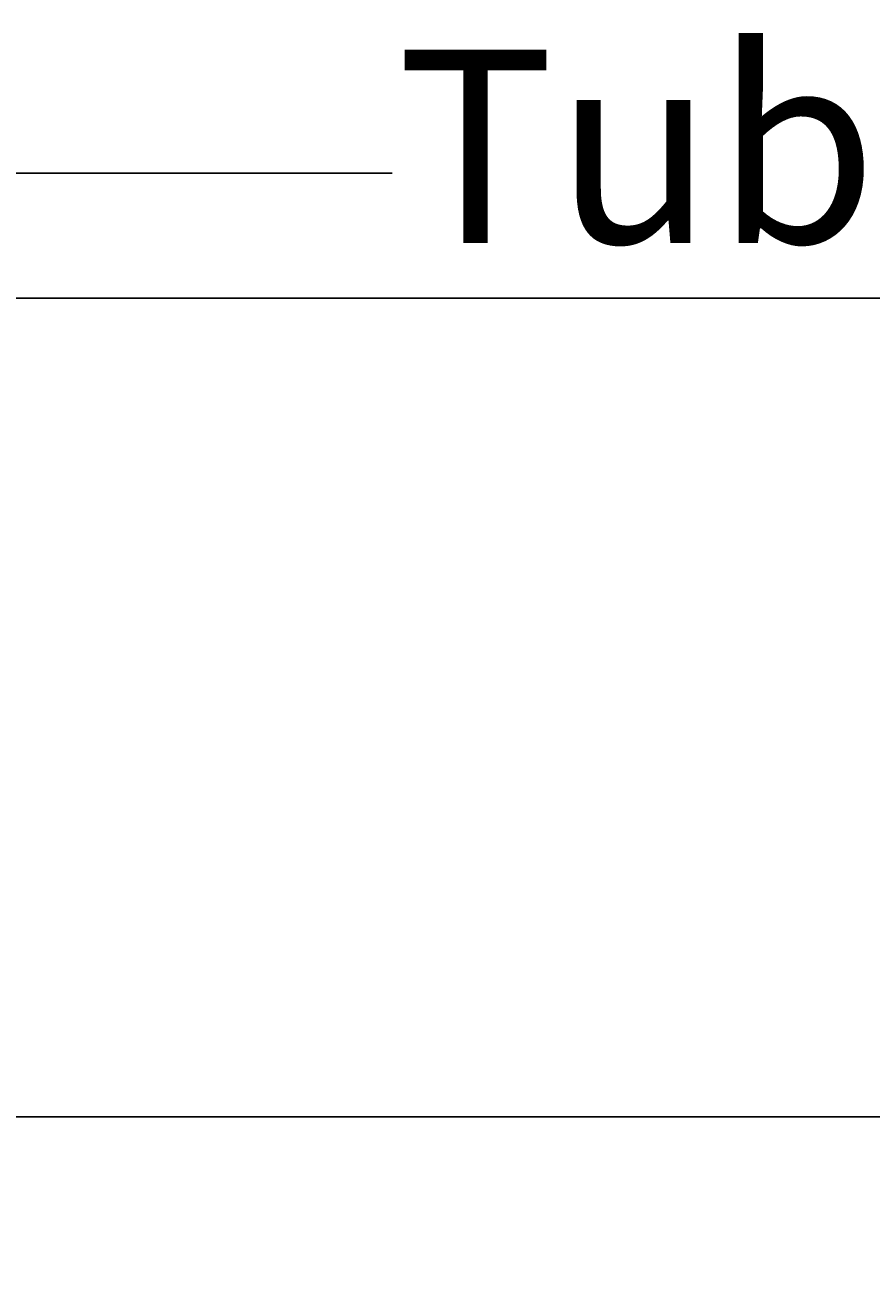
# Model space of a CAD drawing. Units: inches. Extents: x -12 to 334, y -10 to 186.
# Tile 26 of 77: x 88 to 106, y 135 to 160. Entities that reach past the tile are written whole.
import ezdxf
from ezdxf import colors
from ezdxf.entities.mleader import LeaderData, LeaderLine
from ezdxf.math import Vec2, Vec3

# ---------------------------------------------------------------- set-up
doc = ezdxf.new("R2010")
doc.units = ezdxf.units.IN
doc.header["$MEASUREMENT"] = 0
doc.layers.add('M-ANNO-TEXT', color=3, linetype='Continuous', lineweight=25)
doc.layers.add('M-DIMS', color=2, linetype='Continuous', lineweight=18)
doc.styles.get("Standard").update_dxf_attribs({"font": 'arial.ttf'})
doc.dimstyles.get("Standard").update_dxf_attribs({"dimtxt": 0.18, "dimasz": 0.18, "dimexe": 0.18, "dimexo": 0.0625, "dimgap": 0.09, "dimtad": 0, "dimtih": 1, "dimtoh": 1, "dimdec": 4, "dimzin": 0, "dimdsep": 46, "dimtxsty": 'Standard', "dimcen": 0.09, "dimadec": 0, "dimazin": 0, "dimtfac": 1, "dimtdec": 4, "dimtofl": 0, "dimtmove": 0, "dimatfit": 3, "dimfxl": 1, "dimtolj": 1, "dimtzin": 0, "dimarcsym": 0})

# ---------------------------------------------------------------- blocks, each defined once
blk = doc.blocks.new('*D15')
at = {"layer": 'Defpoints', "color": 0, "transparency": 16777216}
for p in [(106.177, 169.385), (86.888, 109.058), (106.177, 102.896)]:
    blk.add_point(p, dxfattribs=at)
at = {"layer": 'M-DIMS', "color": 0, "lineweight": -2, "transparency": 16777216}
for p, q in [((86.888, 109.121), (86.888, 169.565)), ((106.177, 102.958), (106.177, 169.565)), ((87.068, 169.385), (96.147, 169.385)), ((105.997, 169.385), (96.918, 169.385))]:
    blk.add_line(p, q, dxfattribs=at)
at = {"layer": 'M-DIMS', "color": 0, "transparency": 16777216}
for points in [[(87.068, 169.415), (87.068, 169.355), (86.888, 169.385)], [(105.997, 169.415), (105.997, 169.355), (106.177, 169.385)]]:
    blk.add_solid(points, dxfattribs=at)
at = {"layer": 'M-DIMS', "color": 0, "transparency": 16777216, "insert": (96.532, 169.385), "char_height": 0.18, "attachment_point": 5}
blk.add_mtext('\\A1;19.29', dxfattribs=at)
blk = doc.blocks.new('*D22')
at = {"layer": 'Defpoints', "color": 0, "transparency": 16777216}
for p in [(190.342, 154.835), (-11.174, 137.887), (195.342, 137.887)]:
    blk.add_point(p, dxfattribs=at)
at = {"layer": 'M-DIMS', "color": 0, "lineweight": -2, "transparency": 16777216}
for p, q in [((190.28, 154.835), (-11.354, 154.835)), ((-11.174, 154.655), (-11.174, 146.543)), ((-11.174, 138.067), (-11.174, 146.179)), ((195.28, 137.887), (-11.354, 137.887))]:
    blk.add_line(p, q, dxfattribs=at)
at = {"layer": 'M-DIMS', "color": 0, "transparency": 16777216}
for points in [[(-11.204, 154.655), (-11.144, 154.655), (-11.174, 154.835)], [(-11.204, 138.067), (-11.144, 138.067), (-11.174, 137.887)]]:
    blk.add_solid(points, dxfattribs=at)
at = {"layer": 'M-DIMS', "color": 0, "transparency": 16777216, "insert": (-11.174, 146.361), "char_height": 0.18, "attachment_point": 5}
blk.add_mtext('\\A1;16.947', dxfattribs=at)

msp = doc.modelspace()

# ---------------------------------------------------------------- dimensions: what is measured, and where the dimension line sits
at = {"layer": 'M-DIMS'}
dim = msp.add_linear_dim(base=(106.1771, 169.3845), p1=(86.8879, 109.0583), p2=(106.1771, 102.8958), dimstyle='Standard', override={"dimdec": 2, "dimlfac": 1, "dimrnd": 0, "dimzin": 0, "dimdsep": 46, "dimlunit": 2}, dxfattribs=at)
dim.commit()
dim.dimension.update_dxf_attribs({"geometry": '*D15', "text_midpoint": (96.5325, 169.3845)})
dim = msp.add_linear_dim(base=(-11.1736, 137.8871), p1=(190.3421, 154.8345), p2=(195.3421, 137.8871), angle=90, dimstyle='Standard', override={"dimdec": 3, "dimlfac": 1, "dimrnd": 0, "dimzin": 0, "dimdsep": 46, "dimlunit": 2}, dxfattribs=at)
dim.commit()
dim.dimension.update_dxf_attribs({"geometry": '*D22', "text_midpoint": (-11.1735, 146.3608)})

# ---------------------------------------------------------------- leaders
at = {"layer": 'M-ANNO-TEXT'}
ml = msp.add_multileader_mtext('Standard', dxfattribs=at)
ml.set_content('Tube plate', color=256)
ml.set_leader_properties()
ml.build(insert=Vec2(0, 0))
ml.multileader.update_dxf_attribs({"dogleg_length": 0.36, "arrow_head_size": 0.7})
ctx = ml.context
ctx.base_point, ctx.arrow_head_size, ctx.landing_gap_size, ctx.plane_origin = Vec3(95.9742, 157.4218), 0.7, 0.09, Vec3(31.4743, 171.7024)
notes = []
notes.append((ctx, [(0, (1, 1, 0), (78.5354, 157.4218), (1, 0), 17.4388, [(0, [(75.9244, 109.0583)], 0, [])])]))
ctx.mtext.insert, ctx.mtext.flow_direction = Vec3(96.0642, 159.9771), 5
for ctx, leaders in notes:
    for number, flags, end, landing, length, lines in leaders:
        leader = LeaderData()
        leader.index, (leader.has_last_leader_line, leader.has_dogleg_vector, leader.attachment_direction) = number, flags
        leader.last_leader_point, leader.dogleg_vector, leader.dogleg_length = Vec3(end), Vec3(landing), length
        for number, points, colour, breaks in lines:
            line = LeaderLine()
            line.index, line.vertices, line.color, line.breaks = number, Vec3.list(points), colors.encode_raw_color(colour), breaks
            leader.lines.append(line)
        ctx.leaders.append(leader)

doc.saveas('drawing.dxf')
